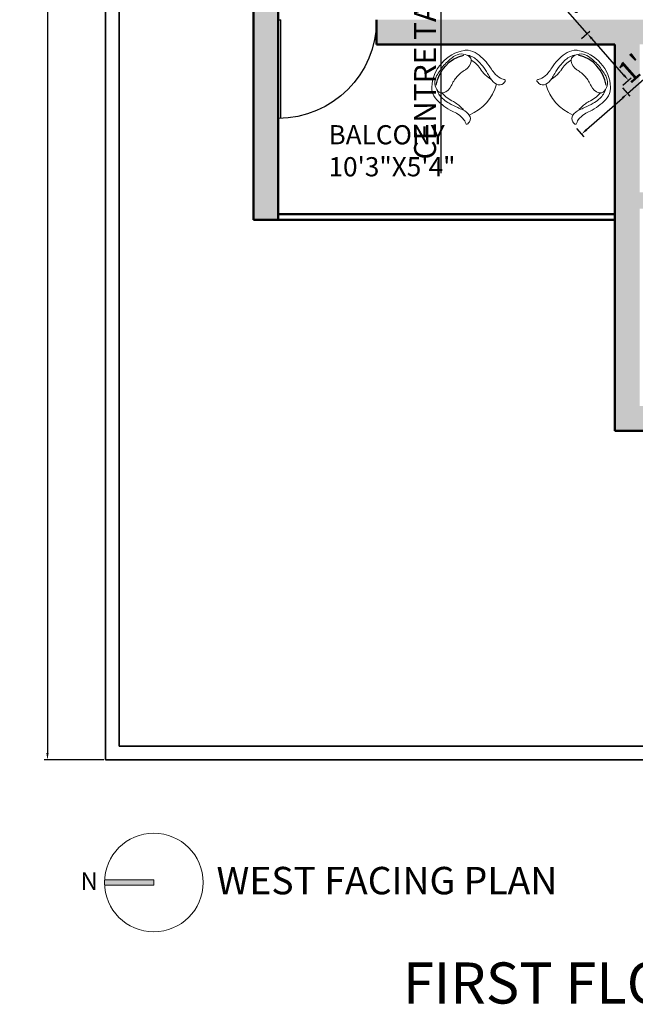
# Model space of a CAD drawing. Units: inches. Extents: x 3008 to 4088, y 1255 to 2137.
# Tile 21 of 30: x 3572 to 3796, y 1260 to 1620. Entities that reach past the tile are written whole.
import ezdxf

# ---------------------------------------------------------------- set-up
doc = ezdxf.new("R2010")
doc.units = ezdxf.units.IN
for name, color, linetype, lineweight in [('A-ANNO-DIMS', 2, 'Continuous', 18), ('A-ANNO-SYMB', 7, 'Continuous', 18), ('A-ANNO-TEXT', 7, 'Continuous', 18), ('A-AREA-IDEN', 7, 'Continuous', 18), ('A-DOOR', 4, 'Continuous', 25), ('A-FURN', 8, 'Continuous', 18), ('A-WALL', 7, 'Continuous', 50), ('A-WALL-PATT', 8, 'Continuous', 13), ('C-PROP', 1, 'Continuous', 35)]:
    doc.layers.add(name, color=color, linetype=linetype, lineweight=lineweight)
doc.layers.add('IFF-FURN-DETAIL', color=250, linetype='Continuous')
doc.styles.get("Standard").update_dxf_attribs({"font": 'arial.ttf'})
doc.dimstyles.new('ISO-25', dxfattribs={"dimtxt": 8, "dimasz": 2.5, "dimexe": 1.25, "dimexo": 0.625, "dimtad": 1, "dimdec": 1, "dimlunit": 3, "dimtxsty": 'Standard', "dimcen": 2.5, "dimadec": 0, "dimazin": 0, "dimtfac": 1, "dimtdec": 1, "dimtmove": 0, "dimatfit": 3, "dimfxl": 1, "dimarcsym": 0})

# ---------------------------------------------------------------- blocks, each defined once
blk = doc.blocks.new('*D32')
at = {"layer": 'A-ANNO-DIMS', "color": 0, "lineweight": -2, "transparency": 16777216}
for p, q in [((3602.32, 2009.72), (3580.54, 2009.72)), ((3581.79, 2007.22), (3581.79, 1352.22)), ((3602.32, 1349.72), (3580.54, 1349.72))]:
    blk.add_line(p, q, dxfattribs=at)
at = {"layer": 'A-ANNO-DIMS', "color": 0, "transparency": 16777216}
for points in [[(3581.37, 2007.22), (3582.2, 2007.22), (3581.79, 2009.72)], [(3581.37, 1352.22), (3582.2, 1352.22), (3581.79, 1349.72)]]:
    blk.add_solid(points, dxfattribs=at)
at = {"layer": 'Defpoints', "color": 0, "transparency": 16777216}
for p in [(3602.94, 2009.72), (3581.79, 1349.72), (3602.94, 1349.72)]:
    blk.add_point(p, dxfattribs=at)
at = {"layer": 'A-ANNO-DIMS', "color": 0, "transparency": 16777216, "insert": (3577.09, 1679.72), "char_height": 8, "attachment_point": 5, "rotation": 90}
blk.add_mtext("55'", dxfattribs=at)
blk = doc.blocks.new('ILNG95')
for points in [[(120, 308, -0.32971), (51, 384, -0.036099), (50, 422, -0.497733), (75, 439, -0.070621), (96, 429, 0.101868), (133, 414, 0.091794), (259, 412, 0.024114), (351, 433, -0.090294), (638, 458, -0.132412), (775, 407, -0.068618), (816, 368, -0.184346), (943, 0, 1.803905)], [(120, 308, 0.138132), (244, 313, 0.001085), (325, 339, -0.034227), (462, 375, -0.033255), (567, 387, -0.137428), (727, 350, -4.561553)], [(120, 308, 0.138132), (244, 313, 0.001085), (325, 339, -0.034227), (462, 375, -0.033255), (567, 387, -0.137428), (727, 350, -4.561553)], [(235, 308, 0.064243), (394, 307, 0.04414), (433, 315, -0.118032), (643, 329, -6.296816)], [(235, 308, 0.064243), (394, 307, 0.04414), (433, 315, -0.118032), (643, 329, -6.296816)], [(639, 0, 0.078302), (612, 161, -0.233633), (633, 315, -0.28763), (710, 349, -0.317923), (875, 193, -0.032882), (900, 0, 1.140397)], [(639, 0, 0.078302), (612, 161, -0.233633), (633, 315, -0.28763), (710, 349, -0.317923), (875, 193, -0.032882), (900, 0, 1.140397)], [(120, -308, 0.32971), (51, -384, 0.036099), (50, -422, 0.497733), (75, -439, 0.070621), (96, -429, -0.101868), (133, -414, -0.091794), (259, -412, -0.024114), (351, -433, 0.090294), (638, -458, 0.132412), (775, -407, 0.068618), (816, -368, 0.184346), (943, 0, -1.803905)], [(639, 0, -0.078302), (612, -161, 0.233633), (633, -315, 0.28763), (710, -349, 0.317923), (875, -193, 0.032882), (900, 0, -1.140397)], [(639, 0, -0.078302), (612, -161, 0.233633), (633, -315, 0.28763), (710, -349, 0.317923), (875, -193, 0.032882), (900, 0, -1.140397)], [(120, -308, -0.138132), (244, -313, -0.001085), (325, -339, 0.034227), (462, -375, 0.033255), (567, -387, 0.137428), (727, -350, 4.561553)], [(120, -308, -0.138132), (244, -313, -0.001085), (325, -339, 0.034227), (462, -375, 0.033255), (567, -387, 0.137428), (727, -350, 4.561553)], [(235, -308, -0.064243), (394, -307, -0.04414), (433, -315, 0.118032), (643, -329, 6.296816)], [(235, -308, -0.064243), (394, -307, -0.04414), (433, -315, 0.118032), (643, -329, 6.296816)]]:
    blk.add_lwpolyline(points, format="xyb")
blk.add_arc((759, 1), 709, 154.3281, 205.801)
at = {"layer": 'IFF-FURN-DETAIL'}
blk.add_arc((326, -2), 549, 326.8997, 34.6691, dxfattribs=at)
blk.add_arc((326, -2), 549, 326.8997, 34.6691, dxfattribs=at)
blk = doc.blocks.new('D1')
for p, q in [((1805.96, 1500.36), (1805.96, 1464.36)), ((1806.96, 1500.36), (1806.96, 1464.36)), ((1805.96, 1464.36), (1806.96, 1464.36))]:
    blk.add_line(p, q)
blk.add_arc((1805.96, 1464.36), 36, 0, 90)
blk = doc.blocks.new('*D51')
at = {"layer": 'A-ANNO-DIMS', "color": 0, "lineweight": -2, "transparency": 16777216}
for p, q in [((3778.81, 1614.68), (3662.79, 1746.22)), ((3776.72, 1612.84), (3779.74, 1615.51)), ((3792.2, 1599.5), (3780.46, 1612.81)), ((3791.76, 1595.78), (3794.79, 1598.45))]:
    blk.add_line(p, q, dxfattribs=at)
at = {"layer": 'A-ANNO-DIMS', "color": 0, "transparency": 16777216}
for points in [[(3780.77, 1613.08), (3780.15, 1612.53), (3778.81, 1614.68)], [(3792.51, 1599.77), (3791.89, 1599.22), (3793.85, 1597.62)]]:
    blk.add_solid(points, dxfattribs=at)
at = {"layer": 'Defpoints', "color": 0, "transparency": 16777216}
for p in [(3778.81, 1614.68), (3776.25, 1612.42), (3791.29, 1595.36)]:
    blk.add_point(p, dxfattribs=at)
at = {"layer": 'A-ANNO-DIMS', "color": 0, "transparency": 16777216, "insert": (3723.54, 1684.54), "char_height": 8, "attachment_point": 5, "rotation": 311.4119}
blk.add_mtext('OUTDOOR CHAIR 1\'-10 1/2" TYP.', dxfattribs=at)
blk = doc.blocks.new('*D52')
at = {"layer": 'A-ANNO-DIMS', "color": 0, "lineweight": -2, "transparency": 16777216}
for p, q in [((3793.55, 1592.8), (3851.01, 1643.48)), ((3791.71, 1594.89), (3794.38, 1591.87)), ((3778.59, 1579.61), (3791.68, 1591.15)), ((3774.87, 1580.05), (3777.54, 1577.02))]:
    blk.add_line(p, q, dxfattribs=at)
at = {"layer": 'A-ANNO-DIMS', "color": 0, "transparency": 16777216}
for points in [[(3791.4, 1591.46), (3791.95, 1590.84), (3793.55, 1592.8)], [(3778.32, 1579.92), (3778.87, 1579.3), (3776.72, 1577.96)]]:
    blk.add_solid(points, dxfattribs=at)
at = {"layer": 'Defpoints', "color": 0, "transparency": 16777216}
for p in [(3791.29, 1595.36), (3793.55, 1592.8), (3774.46, 1580.52)]:
    blk.add_point(p, dxfattribs=at)
at = {"layer": 'A-ANNO-DIMS', "color": 0, "transparency": 16777216, "insert": (3820.07, 1622.54), "char_height": 8, "attachment_point": 5, "rotation": 41.4119}
blk.add_mtext('1\'-10 1/2" TYP.', dxfattribs=at)
blk = doc.blocks.new('*D55')
at = {"layer": 'A-ANNO-DIMS', "color": 0, "lineweight": -2, "transparency": 16777216}
for p, q in [((3721.38, 1734.8), (3726.66, 1734.8)), ((3725.41, 1732.3), (3725.41, 1706.23)), ((3721.38, 1703.73), (3726.66, 1703.73)), ((3725.41, 1703.73), (3725.41, 1563.75))]:
    blk.add_line(p, q, dxfattribs=at)
at = {"layer": 'A-ANNO-DIMS', "color": 0, "transparency": 16777216}
for points in [[(3724.99, 1732.3), (3725.83, 1732.3), (3725.41, 1734.8)], [(3724.99, 1706.23), (3725.83, 1706.23), (3725.41, 1703.73)]]:
    blk.add_solid(points, dxfattribs=at)
at = {"layer": 'Defpoints', "color": 0, "transparency": 16777216}
for p in [(3720.75, 1734.8), (3720.75, 1703.73), (3725.41, 1703.73)]:
    blk.add_point(p, dxfattribs=at)
at = {"layer": 'A-ANNO-DIMS', "color": 0, "transparency": 16777216, "insert": (3720.65, 1632.49), "char_height": 8, "attachment_point": 5, "rotation": 90}
blk.add_mtext('CENTRE TABLE 2\'-7" TYP.', dxfattribs=at)

msp = doc.modelspace()

# ---------------------------------------------------------------- hatches: boundary and pattern name
at = {"layer": 'A-ANNO-SYMB'}
h = msp.add_hatch(color=256, dxfattribs=at)
h.dxf.hatch_style = 1
h.paths.add_polyline_path([(3602.62, 1305.94, 0.013897), (3602.59, 1304.94, 0.013897), (3602.62, 1303.94), (3620.59, 1303.94), (3620.59, 1305.94)])
at = {"layer": 'A-WALL-PATT'}
h = msp.add_hatch(color=256, dxfattribs=at)
h.dxf.hatch_style = 1
h.paths.add_polyline_path([(3665.94, 1631.72), (3656.94, 1631.72), (3656.94, 1546.72), (3665.94, 1546.72)])
h.paths.add_polyline_path([(3851.94, 1619.72), (3701.94, 1619.72), (3701.94, 1610.72), (3788.94, 1610.72), (3788.94, 1469.72), (3809.94, 1469.72), (3809.94, 1478.72), (3797.94, 1478.72), (3797.94, 1550.72), (3815.94, 1550.72), (3815.94, 1556.72), (3797.94, 1556.72), (3797.94, 1610.72), (3845.94, 1610.72), (3845.94, 1586.72), (3851.94, 1586.72)])
h.paths.add_polyline_path([(4028.94, 1631.72), (4019.94, 1631.72), (4019.94, 1619.72), (3887.94, 1619.72), (3887.94, 1610.72), (4019.94, 1610.72), (4019.94, 1577.72), (4028.94, 1577.72)])
h.paths.add_polyline_path([(3875.94, 1478.72), (3851.94, 1478.72), (3851.94, 1556.72), (3845.94, 1556.72), (3845.94, 1526.72), (3845.94, 1478.72), (3833.94, 1478.72), (3833.94, 1469.72), (3875.94, 1469.72)])
h.paths.add_polyline_path([(3959.94, 1478.72), (3917.94, 1478.72), (3917.94, 1469.72), (3959.94, 1469.72)])
h.paths.add_polyline_path([(4028.94, 1511.72), (4019.94, 1511.72), (4019.94, 1478.72), (4001.94, 1478.72), (4001.94, 1469.72), (4028.94, 1469.72)])
h.paths.add_polyline_path([(4028.94, 1699.22), (4019.94, 1699.22), (4019.94, 1673.72), (3893.94, 1673.72), (3893.94, 1649.72), (3899.94, 1649.72), (3899.94, 1667.72), (4019.94, 1667.72), (4019.94, 1655.72), (4028.94, 1655.72)])
h.paths.add_polyline_path([(4028.94, 1847.72), (4019.94, 1847.72), (4019.94, 1796.72), (3863.94, 1796.72), (3863.94, 1790.72), (4019.94, 1790.72), (4019.94, 1765.22), (4028.94, 1765.22)])
h.paths.add_polyline_path([(3815.94, 1796.72), (3779.94, 1796.72), (3665.94, 1796.72), (3665.94, 1898.72), (3656.94, 1898.72), (3656.94, 1673.72), (3665.94, 1673.72), (3665.94, 1790.72), (3815.94, 1790.72)])
h.paths.add_polyline_path([(3755.94, 1949.72), (3656.94, 1949.72), (3656.94, 1940.72), (3665.94, 1940.72), (3755.94, 1940.72)])
h.paths.add_polyline_path([(3827.94, 1949.72), (3797.94, 1949.72), (3797.94, 1940.72), (3809.94, 1940.72), (3809.94, 1874.72), (3815.94, 1874.72), (3815.94, 1940.72), (3827.94, 1940.72)])
h.paths.add_polyline_path([(3953.94, 1949.72), (3851.94, 1949.72), (3851.94, 1940.72), (3863.94, 1940.72), (3863.94, 1844.72), (3809.94, 1844.72), (3809.94, 1832.72), (3815.94, 1832.72), (3815.94, 1838.72), (3863.94, 1838.72), (3869.94, 1838.72), (3869.94, 1940.72), (3953.94, 1940.72)])
h.paths.add_polyline_path([(4028.94, 1949.72), (3995.94, 1949.72), (3995.94, 1940.72), (4019.94, 1940.72), (4019.94, 1889.72), (4028.94, 1889.72)])

# ---------------------------------------------------------------- linework, layer by layer
at = {"layer": 'A-ANNO-SYMB'}
for p, q in [((3620.59, 1305.94), (3602.59, 1305.94)), ((3620.59, 1305.94), (3620.59, 1303.94)), ((3620.59, 1303.94), (3602.59, 1303.94))]:
    msp.add_line(p, q, dxfattribs=at)
msp.add_circle((3620.59, 1304.94), 18, dxfattribs=at)
at = {"layer": 'A-WALL'}
for p, q in [((3656.94, 1546.72), (3656.94, 1949.72)), ((3665.94, 1546.72), (3665.94, 1790.72)), ((3701.94, 1610.72), (3701.94, 1619.72)), ((3701.94, 1610.72), (3788.94, 1610.72)), ((3788.94, 1610.72), (3788.94, 1469.72)), ((3788.94, 1548.72), (3665.94, 1548.72)), ((3788.94, 1546.72), (3656.94, 1546.72)), ((4028.94, 1469.72), (3788.94, 1469.72))]:
    msp.add_line(p, q, dxfattribs=at)
at = {"layer": 'C-PROP'}
for p, q in [((3602.94, 1349.72), (3602.94, 2009.72)), ((3607.94, 1354.72), (3607.94, 2004.72)), ((4077.94, 1354.72), (3607.94, 1354.72)), ((4082.94, 1349.72), (3602.94, 1349.72))]:
    msp.add_line(p, q, dxfattribs=at)

# ---------------------------------------------------------------- block references
at = {"layer": 'A-DOOR', "xscale": -1, "rotation": 180}
msp.add_blockref('D1', (1859.98, 3084.08), dxfattribs=at)
at = {"layer": 'A-FURN', "yscale": 0.0243705291132055, "zscale": 0.0243705291132055}
for p, xscale, rotation in [((3742.93, 1588.62), -0.0243705291132055, 318.5881218623716), ((3766.45, 1588.62), 0.0243705291132055, 41.41187813762839)]:
    msp.add_blockref('ILNG95', p, dxfattribs=dict(at, xscale=xscale, rotation=rotation))

# ---------------------------------------------------------------- texts
at = {"layer": 'A-ANNO-SYMB'}
msp.add_text('N ', height=6.465, dxfattribs=at).set_placement((3593.83, 1302.2))
at = {"layer": 'A-ANNO-TEXT', "attachment_point": 1}
for s, width, insert, char_height in [('{\\fTimes New Roman|b0|i0|c0|p18;WEST FACING PLAN}', 226.7688, (3643.48, 1310.63), 10), ('{\\fTimes New Roman|b0|i0|c0|p18;FIRST FLOOR PLAN}', 294.0396, (3711.51, 1275.76), 15)]:
    msp.add_mtext_dynamic_manual_height_columns(s, width=width, gutter_width=12.5, heights=[0], dxfattribs=dict(at, insert=insert, char_height=char_height))
at = {"layer": 'A-AREA-IDEN', "insert": (3684.38, 1581.24), "char_height": 7, "attachment_point": 1}
msp.add_mtext_dynamic_manual_height_columns('{\\fTimes New Roman|b0|i0|c0|p18;BALCONY\\P10\'3"X5\'4"}', width=105.6127, gutter_width=12.5, heights=[0], dxfattribs=at)

# ---------------------------------------------------------------- dimensions: what is measured, and where the dimension line sits
at = {"layer": 'A-ANNO-DIMS'}
dim = msp.add_linear_dim(base=(3581.79, 1349.72), p1=(3602.94, 2009.72), p2=(3602.94, 1349.72), angle=90, dimstyle='ISO-25', override={"dimclrd": 0, "dimclre": 0, "dimclrt": 0}, dxfattribs=at)
dim.commit()
dim.dimension.update_dxf_attribs({"geometry": '*D32', "text_midpoint": (3577.09, 1679.72)})
for base, p1, p2, angle, text, picture, middle in [((3778.81, 1614.68), (3791.29, 1595.36), (3776.25, 1612.42), 131.4119, 'OUTDOOR CHAIR <> TYP.', '*D51', (3723.54, 1684.54)), ((3725.41, 1703.73), (3720.75, 1734.8), (3720.75, 1703.73), 270, 'CENTRE TABLE <> TYP.', '*D55', (3720.65, 1632.49)), ((3793.55, 1592.8), (3774.46, 1580.52), (3791.29, 1595.36), 41.4119, '<> TYP.', '*D52', (3820.07, 1622.54))]:
    dim = msp.add_linear_dim(base=base, p1=p1, p2=p2, angle=angle, text=text, dimstyle='ISO-25', override={"dimdec": 1, "dimrnd": 0, "dimzin": 1, "dimlunit": 4, "dimfrac": 2}, dxfattribs=at)
    dim.commit()
    dim.dimension.update_dxf_attribs({"geometry": picture, "text_midpoint": middle})

doc.saveas('drawing.dxf')
